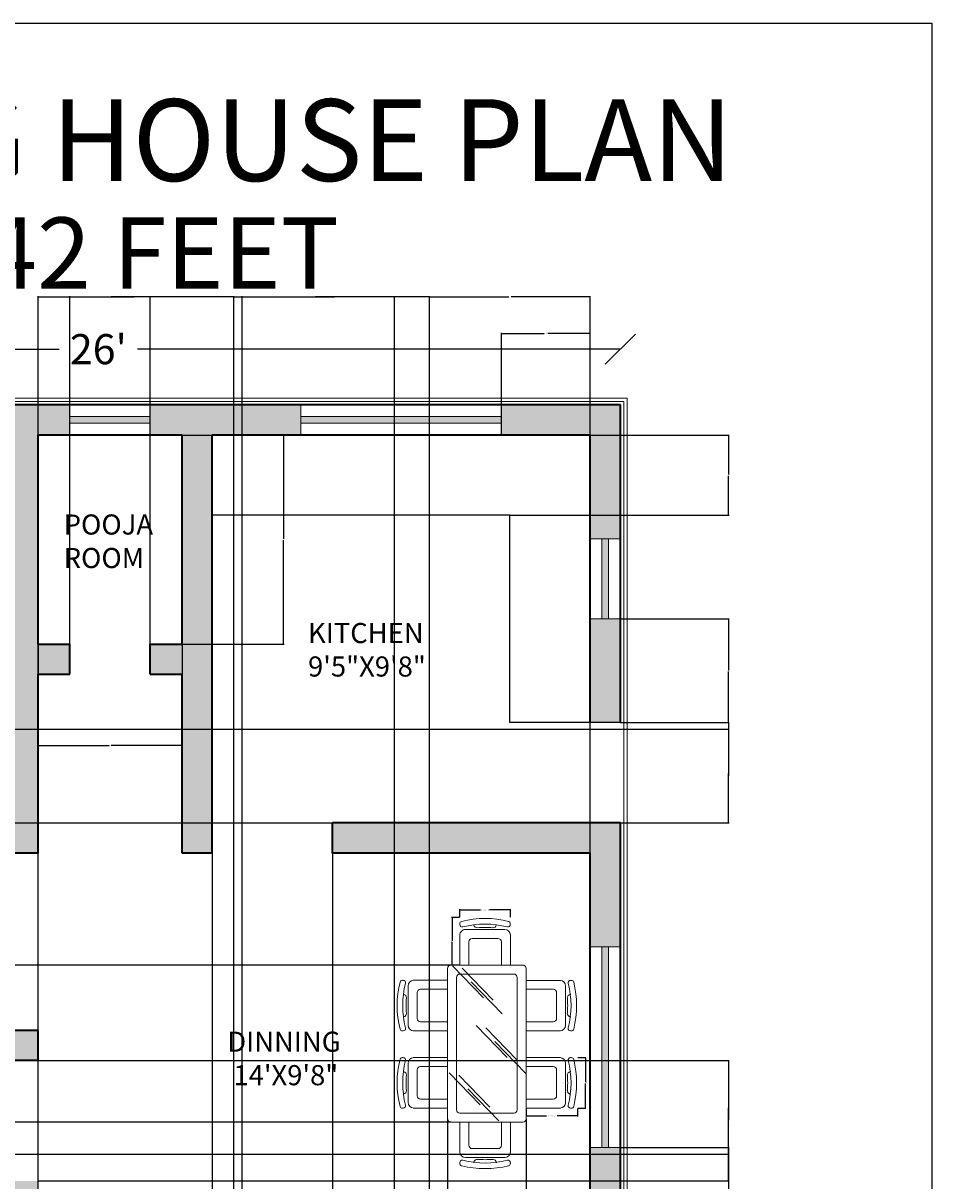
# Model space of a CAD drawing. Units: inches. Extents: x 311 to 815, y -527 to 136.
# Tile 21 of 21: x 544 to 815, y -210 to 136. Entities that reach past the tile are written whole.
import ezdxf

# ---------------------------------------------------------------- set-up
doc = ezdxf.new("R2010")
doc.units = ezdxf.units.IN
doc.header["$MEASUREMENT"] = 0
for name, color, linetype, lineweight in [('A-ANNO-DIMS', 1, 'Continuous', 18), ('A-ANNO-TEXT', 8, 'Continuous', 25), ('A-ANNO-TTLB', 1, 'Continuous', 25), ('A-AREA-IDEN', 8, 'Continuous', 18), ('A-FLOR-CASE', 1, 'Continuous', 25), ('A-FLOR-EDGE', 1, 'Continuous', 18), ('A-GLAZ-PATT', 5, 'Continuous', 13), ('A-WALL-PATT', 242, 'Continuous', 13), ('wall', 1, 'Continuous', 35), ('win', 5, 'Continuous', 18)]:
    doc.layers.add(name, color=color, linetype=linetype, lineweight=lineweight)
doc.layers.add('furniture', color=50, linetype='Continuous', lineweight=13, transparency=0.8)
doc.styles.get("Standard").update_dxf_attribs({"font": 'arial.ttf'})
doc.dimstyles.get("Standard").update_dxf_attribs({"dimtxt": 0.18, "dimasz": 0.18, "dimexe": 0.18, "dimexo": 0.0625, "dimgap": 0.09, "dimtad": 0, "dimtih": 1, "dimtoh": 1, "dimdec": 1, "dimzin": 0, "dimdsep": 46, "dimlunit": 4, "dimtxsty": 'Standard', "dimcen": 0.09, "dimadec": 0, "dimazin": 0, "dimtfac": 1, "dimtdec": 1, "dimtofl": 0, "dimtmove": 0, "dimatfit": 3, "dimfxl": 1, "dimtolj": 1, "dimtzin": 0, "dimarcsym": 0})

# ---------------------------------------------------------------- blocks, each defined once
blk = doc.blocks.new('_ArchTick')
at = {"color": 0, "linetype": 'ByBlock', "const_width": 0.15}
blk.add_lwpolyline([(-0.5, -0.5), (0.5, 0.5)], dxfattribs=at)
blk = doc.blocks.new('_Oblique')
at = {"color": 0, "linetype": 'ByBlock', "lineweight": -2}
blk.add_line((-0.5, -0.5), (0.5, 0.5), dxfattribs=at)
blk = doc.blocks.new('*D2')
at = {"layer": 'A-ANNO-DIMS', "color": 0, "lineweight": -2, "transparency": 16777216}
for p, q in [((410.32, 38.54), (554.61, 38.54)), ((722.32, 38.54), (578.04, 38.54))]:
    blk.add_line(p, q, dxfattribs=at)
at = {"layer": 'Defpoints', "color": 0, "transparency": 16777216}
for p in [(722.32, 38.54), (410.32, 21.87), (722.32, 21.87)]:
    blk.add_point(p, dxfattribs=at)
at = {"layer": 'A-ANNO-DIMS', "color": 0, "lineweight": -2, "transparency": 16777216, "xscale": 9, "yscale": 9, "zscale": 9, "rotation": 180}
blk.add_blockref('_ArchTick', (410.32, 38.54), dxfattribs=at)
at = {"layer": 'A-ANNO-DIMS', "color": 0, "lineweight": -2, "transparency": 16777216, "xscale": 9, "yscale": 9, "zscale": 9}
blk.add_blockref('_Oblique', (722.32, 38.54), dxfattribs=at)
at = {"layer": 'A-ANNO-DIMS', "color": 0, "transparency": 16777216, "insert": (566.32, 38.54), "char_height": 9, "attachment_point": 5}
blk.add_mtext("\\A1;26'", dxfattribs=at)
blk = doc.blocks.new('WIN-60IN')
for p, q in [((9, 60), (0, 60)), ((3.5, 0), (3.5, 60)), ((5.5, 0), (5.5, 60)), ((9, 0), (0, 0))]:
    blk.add_line(p, q)
blk = doc.blocks.new('WIN-24IN')
for p, q in [((9, 24), (0, 24)), ((3.5, 0), (3.5, 24)), ((5.5, 0), (5.5, 24)), ((9, 0), (0, 0))]:
    blk.add_line(p, q)
blk = doc.blocks.new('CHAIR-DINING-SIDE')
for p, q in [((5.18, 15.09), (4.83, 15.09)), ((15.1, 15.09), (4.98, 15.09)), ((1.88, 10.9), (1.78, 10.9)), ((3.31, 13.41), (3.31, 1.68)), ((5.99, 11.4), (5.99, 3.69)), ((15.1, 12.4), (6.99, 12.4)), ((1.88, 4.19), (1.78, 4.19)), ((6.99, 2.68), (15.1, 2.68)), ((4.83, 0), (5.18, 0)), ((4.98, 0), (15.1, 0))]:
    blk.add_line(p, q)
for centre, radius, start, end in [((28.79, 7.54), 28.79, 165.853, 194.147), ((1.52, 14.42), 0.67, 84.0784, 165.853), ((1.7, 16.08), 1.01, 264.0784, 275.9216), ((28.79, 7.54), 27.11, 165.6786, 194.3214), ((1.87, 14.42), 0.67, 345.6786, 95.9216), ((4.98, 13.41), 1.68, 90, 180), ((1.78, 9.89), 1.01, 355.0346, 83.9719), ((6.99, 11.4), 1.01, 90, 180), ((28.79, 7.54), 26.11, 175.0346, 184.9654), ((1.78, 5.2), 1.01, 276.0281, 4.9654), ((6.99, 3.69), 1.01, 180, 270), ((1.52, 0.67), 0.67, 194.147, 275.9216), ((1.7, -1), 1.01, 84.0784, 95.9216), ((1.87, 0.67), 0.67, 264.0784, 14.3214), ((4.98, 1.68), 1.68, 180, 270)]:
    blk.add_arc(centre, radius, start, end)
blk = doc.blocks.new('CHAIR-DINING-END')
for p, q in [((0, 4.98), (0, 13.93)), ((2.68, 6.99), (2.68, 13.93)), ((12.4, 13.93), (12.4, 6.99)), ((15.09, 13.93), (15.09, 4.98)), ((0, 4.83), (0, 5.18)), ((11.4, 5.99), (3.69, 5.99)), ((15.09, 5.18), (15.09, 4.83)), ((13.41, 3.31), (1.68, 3.31)), ((4.19, 1.88), (4.19, 1.78)), ((10.9, 1.88), (10.9, 1.78))]:
    blk.add_line(p, q)
for centre, radius, start, end in [((3.69, 6.99), 1.01, 180, 270), ((11.4, 6.99), 1.01, 270, 0), ((1.68, 4.98), 1.68, 180, 270), ((13.41, 4.98), 1.68, 270, 0), ((0.67, 1.87), 0.67, 75.6786, 185.9216), ((-1, 1.7), 1.01, 354.0784, 5.9216), ((0.67, 1.52), 0.67, 174.0784, 255.853), ((7.54, 28.79), 28.79, 255.853, 284.147), ((7.54, 28.79), 27.11, 255.6786, 284.3214), ((5.2, 1.78), 1.01, 85.0346, 173.9719), ((7.54, 28.79), 26.11, 265.0346, 274.9654), ((9.89, 1.78), 1.01, 6.0281, 94.9654), ((14.42, 1.87), 0.67, 354.0784, 104.3214), ((14.42, 1.52), 0.67, 284.147, 5.9216), ((16.08, 1.7), 1.01, 174.0784, 185.9216)]:
    blk.add_arc(centre, radius, start, end)
blk = doc.blocks.new('*D16')
at = {"layer": 'A-ANNO-DIMS', "color": 0, "lineweight": -2, "transparency": 16777216}
for p, q in [((694.16, -188.46), (694.16, -190.89)), ((709.56, -188.46), (709.56, -190.89)), ((694.34, -190.71), (700.26, -190.71)), ((709.38, -190.71), (703.46, -190.71))]:
    blk.add_line(p, q, dxfattribs=at)
at = {"layer": 'A-ANNO-DIMS', "color": 0, "transparency": 16777216}
for points in [[(694.34, -190.68), (694.34, -190.74), (694.16, -190.71)], [(709.38, -190.68), (709.38, -190.74), (709.56, -190.71)]]:
    blk.add_solid(points, dxfattribs=at)
at = {"layer": 'Defpoints', "color": 0, "transparency": 16777216}
for p in [(694.16, -188.4), (709.56, -188.4), (694.16, -190.71)]:
    blk.add_point(p, dxfattribs=at)
at = {"layer": 'A-ANNO-DIMS', "color": 0, "transparency": 16777216, "insert": (701.86, -190.71), "char_height": 0.18, "attachment_point": 5}
blk.add_mtext('\\A1;SIDE CHAIR 1\'-3 1/2" TYP.', dxfattribs=at)
blk = doc.blocks.new('*D17')
at = {"layer": 'A-ANNO-DIMS', "color": 0, "lineweight": -2, "transparency": 16777216}
for p, q in [((709.62, -173.25), (712.04, -173.25)), ((711.86, -173.43), (711.86, -180.65)), ((711.86, -188.22), (711.86, -181.01)), ((709.62, -188.4), (712.04, -188.4))]:
    blk.add_line(p, q, dxfattribs=at)
at = {"layer": 'A-ANNO-DIMS', "color": 0, "transparency": 16777216}
for points in [[(711.83, -173.43), (711.89, -173.43), (711.86, -173.25)], [(711.83, -188.22), (711.89, -188.22), (711.86, -188.4)]]:
    blk.add_solid(points, dxfattribs=at)
at = {"layer": 'Defpoints', "color": 0, "transparency": 16777216}
for p in [(709.56, -173.25), (709.56, -188.4), (711.86, -188.4)]:
    blk.add_point(p, dxfattribs=at)
at = {"layer": 'A-ANNO-DIMS', "color": 0, "transparency": 16777216, "insert": (711.86, -180.83), "char_height": 0.18, "attachment_point": 5}
blk.add_mtext('\\A1;1\'-3" TYP.', dxfattribs=at)
blk = doc.blocks.new('*D18')
at = {"layer": 'A-ANNO-DIMS', "color": 0, "lineweight": -2, "transparency": 16777216}
for p, q in [((674.33, -131.33), (674.33, -128.94)), ((674.51, -129.12), (680.54, -129.12)), ((689.29, -129.12), (683.26, -129.12)), ((689.47, -131.33), (689.47, -128.94))]:
    blk.add_line(p, q, dxfattribs=at)
at = {"layer": 'A-ANNO-DIMS', "color": 0, "transparency": 16777216}
for points in [[(674.51, -129.09), (674.51, -129.15), (674.33, -129.12)], [(689.29, -129.09), (689.29, -129.15), (689.47, -129.12)]]:
    blk.add_solid(points, dxfattribs=at)
at = {"layer": 'Defpoints', "color": 0, "transparency": 16777216}
for p in [(674.33, -129.12), (674.33, -131.39), (689.47, -131.39)]:
    blk.add_point(p, dxfattribs=at)
at = {"layer": 'A-ANNO-DIMS', "color": 0, "transparency": 16777216, "insert": (681.9, -129.12), "char_height": 0.18, "attachment_point": 5}
blk.add_mtext('\\A1;END CHAIR 1\'-3" TYP.', dxfattribs=at)
blk = doc.blocks.new('*D19')
at = {"layer": 'A-ANNO-DIMS', "color": 0, "lineweight": -2, "transparency": 16777216}
for p, q in [((674.26, -131.39), (671.87, -131.39)), ((672.05, -131.57), (672.05, -138.32)), ((672.05, -145.44), (672.05, -138.69)), ((674.26, -145.62), (671.87, -145.62))]:
    blk.add_line(p, q, dxfattribs=at)
at = {"layer": 'A-ANNO-DIMS', "color": 0, "transparency": 16777216}
for points in [[(672.02, -131.57), (672.08, -131.57), (672.05, -131.39)], [(672.02, -145.44), (672.08, -145.44), (672.05, -145.62)]]:
    blk.add_solid(points, dxfattribs=at)
at = {"layer": 'Defpoints', "color": 0, "transparency": 16777216}
for p in [(674.33, -131.39), (672.05, -145.62), (674.33, -145.62)]:
    blk.add_point(p, dxfattribs=at)
at = {"layer": 'A-ANNO-DIMS', "color": 0, "transparency": 16777216, "insert": (672.05, -138.5), "char_height": 0.18, "attachment_point": 5}
blk.add_mtext('\\A1;1\'-2" TYP.', dxfattribs=at)
blk = doc.blocks.new('*D20')
at = {"layer": 'A-ANNO-DIMS', "color": 0, "lineweight": -2, "transparency": 16777216}
for p, q in [((548.32, -49.69), (548.32, -80.16)), ((591.32, -49.69), (591.32, -80.16)), ((548.5, -79.98), (569.49, -79.98)), ((591.14, -79.98), (570.15, -79.98))]:
    blk.add_line(p, q, dxfattribs=at)
at = {"layer": 'A-ANNO-DIMS', "color": 0, "transparency": 16777216}
for points in [[(548.5, -79.95), (548.5, -80.01), (548.32, -79.98)], [(591.14, -79.95), (591.14, -80.01), (591.32, -79.98)]]:
    blk.add_solid(points, dxfattribs=at)
at = {"layer": 'Defpoints', "color": 0, "transparency": 16777216}
for p in [(548.32, -49.63), (591.32, -49.63), (548.32, -79.98)]:
    blk.add_point(p, dxfattribs=at)
at = {"layer": 'A-ANNO-DIMS', "color": 0, "transparency": 16777216, "insert": (569.82, -79.98), "char_height": 0.18, "attachment_point": 5}
blk.add_mtext('\\A1;3\'-7"', dxfattribs=at)
blk = doc.blocks.new('*D21')
at = {"layer": 'A-ANNO-DIMS', "color": 0, "lineweight": -2, "transparency": 16777216}
for p, q in [((591.39, 12.87), (621.85, 12.87)), ((621.67, 12.69), (621.67, -18.19)), ((621.67, -49.45), (621.67, -18.56)), ((591.39, -49.63), (621.85, -49.63))]:
    blk.add_line(p, q, dxfattribs=at)
at = {"layer": 'A-ANNO-DIMS', "color": 0, "transparency": 16777216}
for points in [[(621.64, 12.69), (621.7, 12.69), (621.67, 12.87)], [(621.64, -49.45), (621.7, -49.45), (621.67, -49.63)]]:
    blk.add_solid(points, dxfattribs=at)
at = {"layer": 'Defpoints', "color": 0, "transparency": 16777216}
for p in [(591.32, 12.87), (591.32, -49.63), (621.67, -49.63)]:
    blk.add_point(p, dxfattribs=at)
at = {"layer": 'A-ANNO-DIMS', "color": 0, "transparency": 16777216, "insert": (621.67, -18.38), "char_height": 0.18, "attachment_point": 5}
blk.add_mtext('\\A1;5\'-2 1/2"', dxfattribs=at)
blk = doc.blocks.new('*D22')
at = {"layer": 'A-ANNO-DIMS', "color": 0, "lineweight": -2, "transparency": 16777216}
for p, q in [((686.89, 12.87), (754.85, 12.87)), ((754.67, 12.69), (754.67, 1.05)), ((754.67, -10.95), (754.67, 0.69)), ((689.39, -11.13), (754.85, -11.13))]:
    blk.add_line(p, q, dxfattribs=at)
at = {"layer": 'A-ANNO-DIMS', "color": 0, "transparency": 16777216}
for points in [[(754.64, 12.69), (754.7, 12.69), (754.67, 12.87)], [(754.64, -10.95), (754.7, -10.95), (754.67, -11.13)]]:
    blk.add_solid(points, dxfattribs=at)
at = {"layer": 'Defpoints', "color": 0, "transparency": 16777216}
for p in [(686.82, 12.87), (689.32, -11.13), (754.67, -11.13)]:
    blk.add_point(p, dxfattribs=at)
at = {"layer": 'A-ANNO-DIMS', "color": 0, "transparency": 16777216, "insert": (754.67, 0.87), "char_height": 0.18, "attachment_point": 5}
blk.add_mtext('\\A1;2\'-0"', dxfattribs=at)
blk = doc.blocks.new('*D25')
at = {"layer": 'A-ANNO-DIMS', "color": 0, "lineweight": -2, "transparency": 16777216}
for p, q in [((606.82, -473.07), (606.82, 54.4)), ((607, 54.22), (630.49, 54.22)), ((654.64, 54.22), (631.16, 54.22)), ((654.82, -473.07), (654.82, 54.4))]:
    blk.add_line(p, q, dxfattribs=at)
at = {"layer": 'A-ANNO-DIMS', "color": 0, "transparency": 16777216}
for points in [[(607, 54.25), (607, 54.19), (606.82, 54.22)], [(654.64, 54.25), (654.64, 54.19), (654.82, 54.22)]]:
    blk.add_solid(points, dxfattribs=at)
at = {"layer": 'Defpoints', "color": 0, "transparency": 16777216}
for p in [(654.82, 54.22), (606.82, -473.13), (654.82, -473.13)]:
    blk.add_point(p, dxfattribs=at)
at = {"layer": 'A-ANNO-DIMS', "color": 0, "transparency": 16777216, "insert": (630.82, 54.22), "char_height": 0.18, "attachment_point": 5}
blk.add_mtext('\\A1;4\'-0"', dxfattribs=at)
blk = doc.blocks.new('*D27')
at = {"layer": 'A-ANNO-DIMS', "color": 0, "lineweight": -2, "transparency": 16777216}
for p, q in [((548.32, -473.07), (548.32, 54.4)), ((548.5, 54.22), (576.96, 54.22)), ((606.64, 54.22), (578.19, 54.22)), ((606.82, -473.07), (606.82, 54.4))]:
    blk.add_line(p, q, dxfattribs=at)
at = {"layer": 'A-ANNO-DIMS', "color": 0, "transparency": 16777216}
for points in [[(548.5, 54.25), (548.5, 54.19), (548.32, 54.22)], [(606.64, 54.25), (606.64, 54.19), (606.82, 54.22)]]:
    blk.add_solid(points, dxfattribs=at)
at = {"layer": 'Defpoints', "color": 0, "transparency": 16777216}
for p in [(606.82, 54.22), (548.32, -473.13), (606.82, -473.13)]:
    blk.add_point(p, dxfattribs=at)
at = {"layer": 'A-ANNO-DIMS', "color": 0, "transparency": 16777216, "insert": (577.57, 54.22), "char_height": 0.18, "attachment_point": 5}
blk.add_mtext('\\A1;4\'-10 1/2"', dxfattribs=at)
blk = doc.blocks.new('*D29')
at = {"layer": 'A-ANNO-DIMS', "color": 0, "lineweight": -2, "transparency": 16777216}
for p, q in [((722.39, -200.13), (754.85, -200.13)), ((754.67, -200.31), (754.67, -231.19)), ((754.67, -262.45), (754.67, -231.56)), ((722.39, -262.63), (754.85, -262.63))]:
    blk.add_line(p, q, dxfattribs=at)
at = {"layer": 'A-ANNO-DIMS', "color": 0, "transparency": 16777216}
for points in [[(754.64, -200.31), (754.7, -200.31), (754.67, -200.13)], [(754.64, -262.45), (754.7, -262.45), (754.67, -262.63)]]:
    blk.add_solid(points, dxfattribs=at)
at = {"layer": 'Defpoints', "color": 0, "transparency": 16777216}
for p in [(722.32, -200.13), (722.32, -262.63), (754.67, -262.63)]:
    blk.add_point(p, dxfattribs=at)
at = {"layer": 'A-ANNO-DIMS', "color": 0, "transparency": 16777216, "insert": (754.67, -231.38), "char_height": 0.18, "attachment_point": 5}
blk.add_mtext('\\A1;5\'-2 1/2"', dxfattribs=at)
blk = doc.blocks.new('*D31')
at = {"layer": 'A-ANNO-DIMS', "color": 0, "lineweight": -2, "transparency": 16777216}
for p, q in [((670.7, -191.61), (670.7, -526.66)), ((694.16, -191.61), (694.16, -526.66)), ((670.88, -526.48), (681.83, -526.48)), ((693.98, -526.48), (683.03, -526.48))]:
    blk.add_line(p, q, dxfattribs=at)
at = {"layer": 'A-ANNO-DIMS', "color": 0, "transparency": 16777216}
for points in [[(670.88, -526.45), (670.88, -526.51), (670.7, -526.48)], [(693.98, -526.45), (693.98, -526.51), (694.16, -526.48)]]:
    blk.add_solid(points, dxfattribs=at)
at = {"layer": 'Defpoints', "color": 0, "transparency": 16777216}
for p in [(670.7, -191.55), (694.16, -191.55), (694.16, -526.48)]:
    blk.add_point(p, dxfattribs=at)
at = {"layer": 'A-ANNO-DIMS', "color": 0, "transparency": 16777216, "insert": (682.43, -526.48), "char_height": 0.18, "attachment_point": 5}
blk.add_mtext('\\A1;1\'-11 1/2"', dxfattribs=at)
blk = doc.blocks.new('*D32')
at = {"layer": 'A-ANNO-DIMS', "color": 0, "lineweight": -2, "transparency": 16777216}
for p, q in [((671.64, -145.62), (377.79, -145.62)), ((377.97, -145.8), (377.97, -168.9)), ((377.97, -192.37), (377.97, -169.27)), ((671.64, -192.55), (377.79, -192.55))]:
    blk.add_line(p, q, dxfattribs=at)
at = {"layer": 'A-ANNO-DIMS', "color": 0, "transparency": 16777216}
for points in [[(377.94, -145.8), (378, -145.8), (377.97, -145.62)], [(377.94, -192.37), (378, -192.37), (377.97, -192.55)]]:
    blk.add_solid(points, dxfattribs=at)
at = {"layer": 'Defpoints', "color": 0, "transparency": 16777216}
for p in [(671.7, -145.62), (377.97, -192.55), (671.7, -192.55)]:
    blk.add_point(p, dxfattribs=at)
at = {"layer": 'A-ANNO-DIMS', "color": 0, "transparency": 16777216, "insert": (377.97, -169.08), "char_height": 0.18, "attachment_point": 5}
blk.add_mtext('\\A1;3\'-11"', dxfattribs=at)
blk = doc.blocks.new('*D35')
at = {"layer": 'A-ANNO-DIMS', "color": 0, "lineweight": -2, "transparency": 16777216}
for p, q in [((665.32, -237.07), (665.32, 54.4)), ((665.5, 54.22), (688.99, 54.22)), ((713.14, 54.22), (689.66, 54.22)), ((713.32, -237.07), (713.32, 54.4))]:
    blk.add_line(p, q, dxfattribs=at)
at = {"layer": 'A-ANNO-DIMS', "color": 0, "transparency": 16777216}
for points in [[(665.5, 54.25), (665.5, 54.19), (665.32, 54.22)], [(713.14, 54.25), (713.14, 54.19), (713.32, 54.22)]]:
    blk.add_solid(points, dxfattribs=at)
at = {"layer": 'Defpoints', "color": 0, "transparency": 16777216}
for p in [(713.32, 54.22), (665.32, -237.13), (713.32, -237.13)]:
    blk.add_point(p, dxfattribs=at)
at = {"layer": 'A-ANNO-DIMS', "color": 0, "transparency": 16777216, "insert": (689.32, 54.22), "char_height": 0.18, "attachment_point": 5}
blk.add_mtext('\\A1;4\'-0"', dxfattribs=at)
blk = doc.blocks.new('*D38')
at = {"layer": 'A-ANNO-DIMS', "color": 0, "lineweight": -2, "transparency": 16777216}
for p, q in [((609.32, -237.07), (609.32, 54.4)), ((609.5, 54.22), (636.99, 54.22)), ((665.14, 54.22), (637.66, 54.22)), ((665.32, -237.07), (665.32, 54.4))]:
    blk.add_line(p, q, dxfattribs=at)
at = {"layer": 'A-ANNO-DIMS', "color": 0, "transparency": 16777216}
for points in [[(609.5, 54.25), (609.5, 54.19), (609.32, 54.22)], [(665.14, 54.25), (665.14, 54.19), (665.32, 54.22)]]:
    blk.add_solid(points, dxfattribs=at)
at = {"layer": 'Defpoints', "color": 0, "transparency": 16777216}
for p in [(665.32, 54.22), (609.32, -237.13), (665.32, -237.13)]:
    blk.add_point(p, dxfattribs=at)
at = {"layer": 'A-ANNO-DIMS', "color": 0, "transparency": 16777216, "insert": (637.32, 54.22), "char_height": 0.18, "attachment_point": 5}
blk.add_mtext('\\A1;4\'-8"', dxfattribs=at)
blk = doc.blocks.new('*D40')
at = {"layer": 'A-ANNO-DIMS', "color": 0, "lineweight": -2, "transparency": 16777216}
for p, q in [((419.39, -75.13), (754.85, -75.13)), ((754.67, -75.31), (754.67, -88.95)), ((754.67, -102.95), (754.67, -89.31)), ((419.39, -103.13), (754.85, -103.13))]:
    blk.add_line(p, q, dxfattribs=at)
at = {"layer": 'A-ANNO-DIMS', "color": 0, "transparency": 16777216}
for points in [[(754.64, -75.31), (754.7, -75.31), (754.67, -75.13)], [(754.64, -102.95), (754.7, -102.95), (754.67, -103.13)]]:
    blk.add_solid(points, dxfattribs=at)
at = {"layer": 'Defpoints', "color": 0, "transparency": 16777216}
for p in [(419.32, -75.13), (419.32, -103.13), (754.67, -103.13)]:
    blk.add_point(p, dxfattribs=at)
at = {"layer": 'A-ANNO-DIMS', "color": 0, "transparency": 16777216, "insert": (754.67, -89.13), "char_height": 0.18, "attachment_point": 5}
blk.add_mtext('\\A1;2\'-4"', dxfattribs=at)
blk = doc.blocks.new('*D42')
at = {"layer": 'A-ANNO-DIMS', "color": 0, "lineweight": -2, "transparency": 16777216}
for p, q in [((419.39, -174.13), (754.85, -174.13)), ((754.67, -174.31), (754.67, -187.95)), ((754.67, -201.95), (754.67, -188.31)), ((419.39, -202.13), (754.85, -202.13))]:
    blk.add_line(p, q, dxfattribs=at)
at = {"layer": 'A-ANNO-DIMS', "color": 0, "transparency": 16777216}
for points in [[(754.64, -174.31), (754.7, -174.31), (754.67, -174.13)], [(754.64, -201.95), (754.7, -201.95), (754.67, -202.13)]]:
    blk.add_solid(points, dxfattribs=at)
at = {"layer": 'Defpoints', "color": 0, "transparency": 16777216}
for p in [(419.32, -174.13), (419.32, -202.13), (754.67, -202.13)]:
    blk.add_point(p, dxfattribs=at)
at = {"layer": 'A-ANNO-DIMS', "color": 0, "transparency": 16777216, "insert": (754.67, -188.13), "char_height": 0.18, "attachment_point": 5}
blk.add_mtext('\\A1;2\'-4"', dxfattribs=at)
blk = doc.blocks.new('*D46')
at = {"layer": 'A-ANNO-DIMS', "color": 0, "lineweight": -2, "transparency": 16777216}
for p, q in [((686.82, 12.93), (686.82, 43.4)), ((687, 43.22), (699.53, 43.22)), ((713.14, 43.22), (700.61, 43.22)), ((713.32, 12.93), (713.32, 43.4))]:
    blk.add_line(p, q, dxfattribs=at)
at = {"layer": 'A-ANNO-DIMS', "color": 0, "transparency": 16777216}
for points in [[(687, 43.25), (687, 43.19), (686.82, 43.22)], [(713.14, 43.25), (713.14, 43.19), (713.32, 43.22)]]:
    blk.add_solid(points, dxfattribs=at)
at = {"layer": 'Defpoints', "color": 0, "transparency": 16777216}
for p in [(713.32, 43.22), (686.82, 12.87), (713.32, 12.87)]:
    blk.add_point(p, dxfattribs=at)
at = {"layer": 'A-ANNO-DIMS', "color": 0, "transparency": 16777216, "insert": (700.07, 43.22), "char_height": 0.18, "attachment_point": 5}
blk.add_mtext('\\A1;2\'-2 1/2"', dxfattribs=at)
blk = doc.blocks.new('*D47')
at = {"layer": 'A-ANNO-DIMS', "color": 0, "lineweight": -2, "transparency": 16777216}
for p, q in [((722.39, -42.13), (754.85, -42.13)), ((754.67, -42.31), (754.67, -57.45)), ((754.67, -72.95), (754.67, -57.81)), ((722.39, -73.13), (754.85, -73.13))]:
    blk.add_line(p, q, dxfattribs=at)
at = {"layer": 'A-ANNO-DIMS', "color": 0, "transparency": 16777216}
for points in [[(754.64, -42.31), (754.7, -42.31), (754.67, -42.13)], [(754.64, -72.95), (754.7, -72.95), (754.67, -73.13)]]:
    blk.add_solid(points, dxfattribs=at)
at = {"layer": 'Defpoints', "color": 0, "transparency": 16777216}
for p in [(722.32, -42.13), (722.32, -73.13), (754.67, -73.13)]:
    blk.add_point(p, dxfattribs=at)
at = {"layer": 'A-ANNO-DIMS', "color": 0, "transparency": 16777216, "insert": (754.67, -57.63), "char_height": 0.18, "attachment_point": 5}
blk.add_mtext('\\A1;2\'-7"', dxfattribs=at)
blk = doc.blocks.new('*D48')
at = {"layer": 'A-ANNO-DIMS', "color": 0, "lineweight": -2, "transparency": 16777216}
for p, q in [((722.39, -73.13), (754.85, -73.13)), ((754.67, -73.31), (754.67, -87.95)), ((754.67, -102.95), (754.67, -88.31)), ((722.39, -103.13), (754.85, -103.13))]:
    blk.add_line(p, q, dxfattribs=at)
at = {"layer": 'A-ANNO-DIMS', "color": 0, "transparency": 16777216}
for points in [[(754.64, -73.31), (754.7, -73.31), (754.67, -73.13)], [(754.64, -102.95), (754.7, -102.95), (754.67, -103.13)]]:
    blk.add_solid(points, dxfattribs=at)
at = {"layer": 'Defpoints', "color": 0, "transparency": 16777216}
for p in [(722.32, -73.13), (722.32, -103.13), (754.67, -103.13)]:
    blk.add_point(p, dxfattribs=at)
at = {"layer": 'A-ANNO-DIMS', "color": 0, "transparency": 16777216, "insert": (754.67, -88.13), "char_height": 0.18, "attachment_point": 5}
blk.add_mtext('\\A1;2\'-6"', dxfattribs=at)
blk = doc.blocks.new('*D49')
at = {"layer": 'A-ANNO-DIMS', "color": 0, "lineweight": -2, "transparency": 16777216}
for p, q in [((600.32, -112.19), (600.32, -526.66)), ((636.32, -112.19), (636.32, -526.66)), ((600.5, -526.48), (617.99, -526.48)), ((636.14, -526.48), (618.65, -526.48))]:
    blk.add_line(p, q, dxfattribs=at)
at = {"layer": 'A-ANNO-DIMS', "color": 0, "transparency": 16777216}
for points in [[(600.5, -526.45), (600.5, -526.51), (600.32, -526.48)], [(636.14, -526.45), (636.14, -526.51), (636.32, -526.48)]]:
    blk.add_solid(points, dxfattribs=at)
at = {"layer": 'Defpoints', "color": 0, "transparency": 16777216}
for p in [(600.32, -112.13), (636.32, -112.13), (636.32, -526.48)]:
    blk.add_point(p, dxfattribs=at)
at = {"layer": 'A-ANNO-DIMS', "color": 0, "transparency": 16777216, "insert": (618.32, -526.48), "char_height": 0.18, "attachment_point": 5}
blk.add_mtext('\\A1;3\'-0"', dxfattribs=at)
blk = doc.blocks.new('*D50')
at = {"layer": 'A-ANNO-DIMS', "color": 0, "lineweight": -2, "transparency": 16777216}
for p, q in [((557.82, -49.57), (557.82, 54.4)), ((558, 54.22), (569.49, 54.22)), ((581.64, 54.22), (570.15, 54.22)), ((581.82, -49.57), (581.82, 54.4))]:
    blk.add_line(p, q, dxfattribs=at)
at = {"layer": 'A-ANNO-DIMS', "color": 0, "transparency": 16777216}
for points in [[(558, 54.25), (558, 54.19), (557.82, 54.22)], [(581.64, 54.25), (581.64, 54.19), (581.82, 54.22)]]:
    blk.add_solid(points, dxfattribs=at)
at = {"layer": 'Defpoints', "color": 0, "transparency": 16777216}
for p in [(581.82, 54.22), (557.82, -49.63), (581.82, -49.63)]:
    blk.add_point(p, dxfattribs=at)
at = {"layer": 'A-ANNO-DIMS', "color": 0, "transparency": 16777216, "insert": (569.82, 54.22), "char_height": 0.18, "attachment_point": 5}
blk.add_mtext('\\A1;2\'-0"', dxfattribs=at)
blk = doc.blocks.new('*D52')
at = {"layer": 'A-ANNO-DIMS', "color": 0, "lineweight": -2, "transparency": 16777216}
for p, q in [((548.39, -174.13), (754.85, -174.13)), ((754.67, -174.31), (754.67, -191.95)), ((754.67, -209.95), (754.67, -192.31)), ((548.39, -210.13), (754.85, -210.13))]:
    blk.add_line(p, q, dxfattribs=at)
at = {"layer": 'A-ANNO-DIMS', "color": 0, "transparency": 16777216}
for points in [[(754.64, -174.31), (754.7, -174.31), (754.67, -174.13)], [(754.64, -209.95), (754.7, -209.95), (754.67, -210.13)]]:
    blk.add_solid(points, dxfattribs=at)
at = {"layer": 'Defpoints', "color": 0, "transparency": 16777216}
for p in [(548.32, -174.13), (548.32, -210.13), (754.67, -210.13)]:
    blk.add_point(p, dxfattribs=at)
at = {"layer": 'A-ANNO-DIMS', "color": 0, "transparency": 16777216, "insert": (754.67, -192.13), "char_height": 0.18, "attachment_point": 5}
blk.add_mtext('\\A1;3\'-0"', dxfattribs=at)

msp = doc.modelspace()

# ---------------------------------------------------------------- hatches: boundary and pattern name
at = {"layer": 'A-GLAZ-PATT'}
h = msp.add_hatch(color=256, dxfattribs=at)
h.dxf.hatch_style = 1
h.paths.add_polyline_path([(415.82, -202.13), (413.82, -202.13), (413.82, -262.13), (415.82, -262.13)])
h.paths.add_polyline_path([(415.82, -390.84), (413.82, -390.84), (413.82, -450.84), (415.82, -450.84)])
h.paths.add_polyline_path([(415.82, -311.57), (413.82, -311.57), (413.82, -335.57), (415.82, -335.57)])
h.paths.add_polyline_path([(509.32, -476.63), (449.32, -476.63), (449.32, -478.63), (509.32, -478.63)])
h.paths.add_polyline_path([(606.82, -476.63), (582.82, -476.63), (582.82, -478.63), (606.82, -478.63)])
h.paths.add_polyline_path([(678.82, -476.63), (654.82, -476.63), (654.82, -478.63), (678.82, -478.63)])
h.paths.add_polyline_path([(718.82, -385.13), (716.82, -385.13), (716.82, -445.13), (718.82, -445.13)])
h.paths.add_polyline_path([(718.82, -262.63), (716.82, -262.63), (716.82, -322.63), (718.82, -322.63)])
h.paths.add_polyline_path([(718.82, -140.13), (716.82, -140.13), (716.82, -200.13), (718.82, -200.13)])
h.paths.add_polyline_path([(718.82, -18.13), (716.82, -18.13), (716.82, -42.13), (718.82, -42.13)])
h.paths.add_polyline_path([(686.82, 18.37), (626.82, 18.37), (626.82, 16.37), (686.82, 16.37)])
h.paths.add_polyline_path([(581.82, 18.37), (557.82, 18.37), (557.82, 16.37), (581.82, 16.37)])
h.paths.add_polyline_path([(509.32, 18.37), (449.32, 18.37), (449.32, 16.37), (509.32, 16.37)])
at = {"layer": 'A-WALL-PATT'}
h = msp.add_hatch(color=256, dxfattribs=at)
h.dxf.hatch_style = 1
h.paths.add_polyline_path([(557.82, 21.87), (509.32, 21.87), (509.32, 12.87), (539.32, 12.87), (539.32, -112.13), (548.32, -112.13), (548.32, -58.63), (557.82, -58.63), (557.82, -49.63), (548.32, -49.63), (548.32, 12.87), (557.82, 12.87)])
h.paths.add_polyline_path([(449.32, 21.87), (410.32, 21.87), (410.32, -15.13), (419.32, -15.13), (419.32, 12.87), (449.32, 12.87)])
h.paths.add_polyline_path([(626.82, 21.87), (581.82, 21.87), (581.82, 12.87), (591.32, 12.87), (591.32, -49.63), (581.82, -49.63), (581.82, -58.63), (591.32, -58.63), (591.32, -112.13), (600.32, -112.13), (600.32, 12.87), (626.82, 12.87)])
h.paths.add_polyline_path([(722.32, 21.87), (686.82, 21.87), (686.82, 12.87), (713.32, 12.87), (713.32, -18.13), (722.32, -18.13)])
h.paths.add_polyline_path([(722.32, -42.13), (713.32, -42.13), (713.32, -73.13), (722.32, -73.13)])
h.paths.add_polyline_path([(501.32, -103.13), (419.32, -103.13), (419.32, -75.13), (410.32, -75.13), (410.32, -126.63), (419.32, -126.63), (419.32, -112.13), (492.32, -112.13), (492.32, -143.13), (501.32, -143.13)])
h.paths.add_polyline_path([(548.32, -165.13), (419.32, -165.13), (419.32, -150.63), (410.32, -150.63), (410.32, -202.13), (419.32, -202.13), (419.32, -174.13), (548.32, -174.13)])
h.paths.add_polyline_path([(722.32, -103.13), (636.32, -103.13), (636.32, -112.13), (713.32, -112.13), (713.32, -140.13), (722.32, -140.13)])
h.paths.add_polyline_path([(548.32, -210.13), (539.32, -210.13), (539.32, -290.13), (419.32, -290.13), (419.32, -262.13), (410.32, -262.13), (410.32, -311.57), (419.32, -311.57), (419.32, -299.13), (469.32, -299.13), (469.32, -348.13), (443.32, -348.13), (443.32, -357.13), (478.32, -357.13), (478.32, -299.13), (548.32, -299.13)])
h.paths.add_polyline_path([(722.32, -200.13), (713.32, -200.13), (713.32, -228.13), (609.32, -228.13), (609.32, -237.13), (713.32, -237.13), (713.32, -262.63), (722.32, -262.63)])
h.paths.add_polyline_path([(722.32, -322.63), (713.32, -322.63), (713.32, -348.13), (633.32, -348.13), (633.32, -357.13), (713.32, -357.13), (713.32, -385.13), (722.32, -385.13)])
h.paths.add_polyline_path([(419.32, -335.57), (410.32, -335.57), (410.32, -390.84), (419.32, -390.84)])
h.paths.add_polyline_path([(419.32, -450.84), (410.32, -450.84), (410.32, -482.13), (449.32, -482.13), (449.32, -473.13), (419.32, -473.13)])
h.paths.add_polyline_path([(582.82, -473.13), (548.32, -473.13), (548.32, -348.13), (539.32, -348.13), (539.32, -473.13), (509.32, -473.13), (509.32, -482.13), (582.82, -482.13)])
h.paths.add_polyline_path([(722.32, -445.13), (713.32, -445.13), (713.32, -473.13), (678.82, -473.13), (678.82, -482.13), (722.32, -482.13)])

# ---------------------------------------------------------------- linework, layer by layer
at = {"layer": 'A-ANNO-TTLB'}
msp.add_lwpolyline([(310.67, 136.01), (815.43, 136.01), (815.43, -506.97), (310.67, -506.97)], close=True, dxfattribs=at)
at = {"layer": 'A-FLOR-CASE'}
for p, q in [((689.32, -11.13), (600.32, -11.13)), ((689.32, -73.13), (689.32, -11.13)), ((722.32, -73.13), (689.32, -73.13))]:
    msp.add_line(p, q, dxfattribs=at)
at = {"layer": 'A-FLOR-EDGE'}
for p, q in [((724.32, 23.87), (408.32, 23.87)), ((723.32, 22.87), (409.32, 22.87)), ((723.32, -483.13), (723.32, 22.87)), ((724.32, -484.13), (724.32, 23.87))]:
    msp.add_line(p, q, dxfattribs=at)
at = {"layer": 'furniture'}
for p, q in [((670.7, -146.62), (670.7, -191.55)), ((693.16, -145.62), (671.7, -145.62)), ((672.16, -145.83), (681.45, -155.43)), ((690.48, -148.3), (674.38, -148.3)), ((675.06, -146.5), (684.35, -156.09)), ((694.16, -191.55), (694.16, -146.62)), ((673.38, -149.3), (673.38, -188.86)), ((677.76, -150.58), (687.04, -160.17)), ((691.48, -188.86), (691.48, -149.3)), ((679.24, -163.69), (688.53, -173.28)), ((682.13, -164.36), (691.42, -173.95)), ((684.83, -168.44), (694.12, -178.03)), ((671.13, -177.86), (680.42, -187.45)), ((674.03, -178.52), (683.31, -188.12)), ((676.72, -182.6), (686.01, -192.2)), ((674.38, -189.87), (690.48, -189.87)), ((671.7, -192.55), (693.16, -192.55))]:
    msp.add_line(p, q, dxfattribs=at)
for centre, radius, start, end in [((671.65, -146.57), 0.959, 87.166, 182.834), ((674.38, -149.3), 1.01, 90, 180), ((690.48, -149.3), 1.01, 0, 90), ((693.16, -146.62), 1.01, 0, 90), ((674.38, -188.86), 1.01, 180, 270), ((690.48, -188.86), 1.01, 270, 0), ((671.7, -191.55), 1.01, 180, 270), ((693.16, -191.55), 1.01, 270, 0)]:
    msp.add_arc(centre, radius, start, end, dxfattribs=at)
at = {"layer": 'wall'}
for p, q in [((722.32, 21.87), (410.32, 21.87)), ((722.32, -73.13), (722.32, 21.87)), ((548.32, -49.63), (548.32, 12.87)), ((548.32, -49.63), (548.32, 12.87)), ((591.32, 12.87), (548.32, 12.87)), ((591.32, -49.63), (591.32, 12.87)), ((713.32, 12.87), (600.32, 12.87)), ((600.32, -112.13), (600.32, 12.87)), ((713.32, -73.13), (713.32, 12.87)), ((548.32, -49.63), (557.82, -49.63)), ((557.82, -58.63), (557.82, -49.63)), ((581.82, -58.63), (581.82, -49.63)), ((581.82, -49.63), (591.32, -49.63)), ((548.32, -112.13), (548.32, -58.63)), ((548.32, -112.13), (548.32, -58.63)), ((548.32, -58.63), (557.82, -58.63)), ((581.82, -58.63), (591.32, -58.63)), ((591.32, -112.13), (591.32, -58.63)), ((722.32, -103.13), (636.32, -103.13)), ((636.32, -112.13), (636.32, -103.13)), ((722.32, -482.13), (722.32, -103.13)), ((548.32, -112.13), (539.32, -112.13)), ((600.32, -112.13), (591.32, -112.13)), ((713.32, -112.13), (636.32, -112.13)), ((713.32, -228.13), (713.32, -112.13)), ((548.32, -165.13), (419.32, -165.13)), ((548.32, -174.13), (548.32, -165.13)), ((548.32, -174.13), (419.32, -174.13))]:
    msp.add_line(p, q, dxfattribs=at)

# ---------------------------------------------------------------- block references
at = {"layer": 'furniture', "rotation": 180}
for name, p in [('CHAIR-DINING-END', (689.44, -131.68)), ('CHAIR-DINING-SIDE', (709.26, -150.18)), ('CHAIR-DINING-SIDE', (709.26, -173.29))]:
    msp.add_blockref(name, p, dxfattribs=at)
at = {"layer": 'furniture'}
for name, p in [('CHAIR-DINING-SIDE', (655.6, -165.26)), ('CHAIR-DINING-SIDE', (655.6, -188.37)), ('CHAIR-DINING-END', (674.36, -206.48))]:
    msp.add_blockref(name, p, dxfattribs=at)
at = {"layer": 'win', "rotation": 90.00000000000003}
for name, p in [('WIN-24IN', (581.82, 12.87)), ('WIN-60IN', (686.82, 12.87))]:
    msp.add_blockref(name, p, dxfattribs=at)
at = {"layer": 'win'}
for name, p in [('WIN-24IN', (713.32, -42.13)), ('WIN-60IN', (713.32, -200.13))]:
    msp.add_blockref(name, p, dxfattribs=at)

# ---------------------------------------------------------------- texts
at = {"layer": 'A-ANNO-TEXT', "attachment_point": 1}
for s, width, gutter_width, insert, char_height in [('EAST FACING HOUSE PLAN ', 457.2415, 4.08, (340.62, 113.27), 24.4528), ('26X42 FEET', 176.1888, 3.55, (483, 77.92), 21.281)]:
    msp.add_mtext_dynamic_manual_height_columns(s, width=width, gutter_width=gutter_width, heights=[0], dxfattribs=dict(at, insert=insert, char_height=char_height))
at = {"layer": 'A-AREA-IDEN', "attachment_point": 1}
for s, width, insert, char_height in [('POOJA ROOM', 30.2489, (555.93, -10.89), 6.007), ('    KITCHEN\\P    9\'5"X9\'8"', 54.4429, (621.63, -43.33), 6.0073), ('    DINNING\\P     14\'X9\'8"', 54.4429, (597.5, -165.52), 6.0073)]:
    msp.add_mtext_dynamic_manual_height_columns(s, width=width, gutter_width=1, heights=[0], dxfattribs=dict(at, insert=insert, char_height=char_height))

# ---------------------------------------------------------------- dimensions: what is measured, and where the dimension line sits
at = {"layer": 'A-ANNO-DIMS'}
for base, p1, p2, override, picture, middle in [((606.82, 54.22), (548.32, -473.13), (606.82, -473.13), {"dimdec": 1, "dimlfac": 1, "dimrnd": 0, "dimzin": 1, "dimdsep": 46, "dimlunit": 4, "dimfrac": 2}, '*D27', (577.57, 54.22)), ((581.82, 54.22), (557.82, -49.63), (581.82, -49.63), {"dimdec": 1, "dimlfac": 1, "dimrnd": 0, "dimzin": 1, "dimdsep": 46, "dimlunit": 4, "dimfrac": 2}, '*D50', (569.82, 54.22)), ((654.82, 54.22), (606.82, -473.13), (654.82, -473.13), {"dimdec": 1, "dimlfac": 1, "dimrnd": 0, "dimzin": 1, "dimdsep": 46, "dimlunit": 4, "dimfrac": 2}, '*D25', (630.82, 54.22)), ((665.32, 54.22), (609.32, -237.13), (665.32, -237.13), {"dimdec": 1, "dimlfac": 1, "dimrnd": 0, "dimzin": 1, "dimdsep": 46, "dimlunit": 4, "dimfrac": 2}, '*D38', (637.32, 54.22)), ((713.32, 54.22), (665.32, -237.13), (713.32, -237.13), {"dimdec": 1, "dimlfac": 1, "dimrnd": 0, "dimzin": 1, "dimdsep": 46, "dimlunit": 4, "dimfrac": 2}, '*D35', (689.32, 54.22)), ((722.32, 38.54), (410.32, 21.87), (722.32, 21.87), {"dimtxt": 9, "dimasz": 9, "dimgap": 4, "dimblk1": 'ArchTick', "dimblk2": 'Oblique', "dimsah": 1, "dimse1": 1, "dimse2": 1, "dimclrd": 0, "dimclre": 0, "dimclrt": 0}, '*D2', (566.32, 38.54)), ((636.32, -526.48), (600.32, -112.13), (636.32, -112.13), {"dimdec": 1, "dimlfac": 1, "dimrnd": 0, "dimzin": 1, "dimdsep": 46, "dimlunit": 4, "dimfrac": 2}, '*D49', (618.32, -526.48)), ((694.16, -526.48), (670.7, -191.55), (694.16, -191.55), {"dimdec": 1, "dimlfac": 1, "dimrnd": 0, "dimzin": 1, "dimdsep": 46, "dimlunit": 4, "dimfrac": 2}, '*D31', (682.43, -526.48))]:
    dim = msp.add_linear_dim(base=base, p1=p1, p2=p2, dimstyle='Standard', override=override, dxfattribs=at)
    dim.commit()
    dim.dimension.update_dxf_attribs({"geometry": picture, "text_midpoint": middle})
for base, p1, p2, angle, picture, middle in [((713.32, 43.22), (686.82, 12.87), (713.32, 12.87), 0, '*D46', (700.07, 43.22)), ((621.67, -49.63), (591.32, 12.87), (591.32, -49.63), 270, '*D21', (621.67, -18.38)), ((754.67, -11.13), (686.82, 12.87), (689.32, -11.13), 90, '*D22', (754.67, 0.87)), ((754.67, -73.13), (722.32, -42.13), (722.32, -73.13), 90, '*D47', (754.67, -57.63)), ((548.32, -79.98), (591.32, -49.63), (548.32, -49.63), 180, '*D20', (569.82, -79.98)), ((754.67, -103.13), (419.32, -75.13), (419.32, -103.13), 90, '*D40', (754.67, -89.13)), ((754.67, -103.13), (722.32, -73.13), (722.32, -103.13), 90, '*D48', (754.67, -88.13)), ((377.97, -192.55), (671.7, -145.62), (671.7, -192.55), 90, '*D32', (377.97, -169.08)), ((754.67, -202.13), (419.32, -174.13), (419.32, -202.13), 90, '*D42', (754.67, -188.13)), ((754.67, -210.13), (548.32, -174.13), (548.32, -210.13), 90, '*D52', (754.67, -192.13)), ((754.67, -262.63), (722.32, -200.13), (722.32, -262.63), 90, '*D29', (754.67, -231.38))]:
    dim = msp.add_linear_dim(base=base, p1=p1, p2=p2, angle=angle, dimstyle='Standard', override={"dimdec": 1, "dimlfac": 1, "dimrnd": 0, "dimzin": 1, "dimdsep": 46, "dimlunit": 4, "dimfrac": 2}, dxfattribs=at)
    dim.commit()
    dim.dimension.update_dxf_attribs({"geometry": picture, "text_midpoint": middle})
for base, p1, p2, angle, text, picture, middle in [((672.05, -145.62), (674.33, -131.39), (674.33, -145.62), 270, '<> TYP.', '*D19', (672.05, -138.5)), ((674.33, -129.12), (689.47, -131.39), (674.33, -131.39), 180, 'END CHAIR <> TYP.', '*D18', (681.9, -129.12)), ((711.864, -188.4022), (709.5553, -173.2544), (709.5553, -188.4022), 270, '<> TYP.', '*D17', (711.864, -180.8283)), ((694.16, -190.71), (709.56, -188.4), (694.16, -188.4), 180, 'SIDE CHAIR <> TYP.', '*D16', (701.86, -190.71))]:
    dim = msp.add_linear_dim(base=base, p1=p1, p2=p2, angle=angle, text=text, dimstyle='Standard', override={"dimdec": 1, "dimlfac": 1, "dimrnd": 0, "dimzin": 1, "dimdsep": 46, "dimlunit": 4, "dimfrac": 2}, dxfattribs=at)
    dim.commit()
    dim.dimension.update_dxf_attribs({"geometry": picture, "text_midpoint": middle})

doc.saveas('drawing.dxf')
